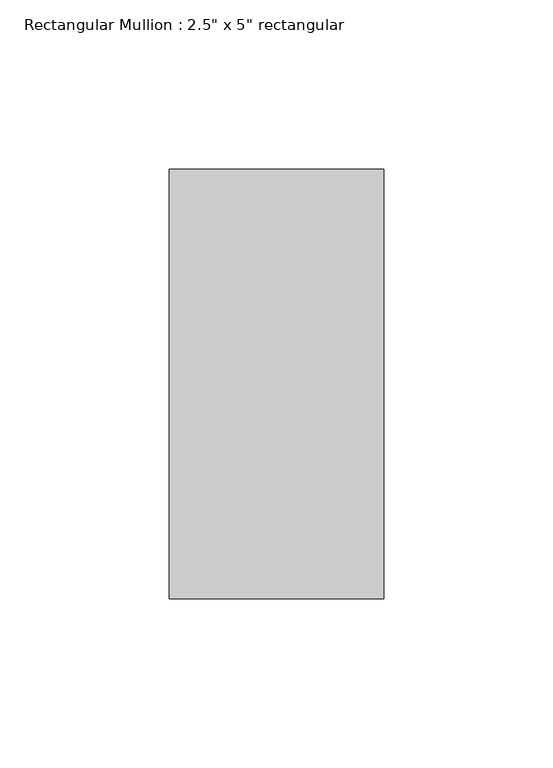
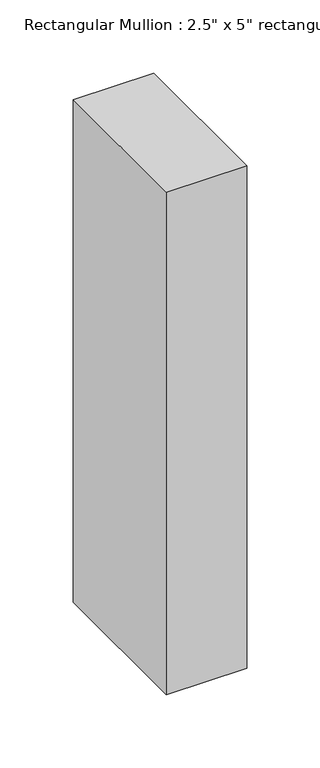
"""IFC4 building model written with IfcOpenShell, lengths in millimetres: member geometry."""

from ifc_helpers import new_model, si_unit, frame, origin, place, context, project, spatial, polyline, outline, extrude, source, transform, mapped, element, save


def member_05170f4c(model_context):
    return source(origin(), model_context, "Body", "SweptSolid", [
        extrude(outline(polyline([(0.0, 63.5), (0.0, -63.5), (-63.5, -63.5), (-63.5, 63.5), (0.0, 63.5)])), frame((0.0, 0.0, -419.0669271), z_axis=(0.0, 0.0, 1.0), x_axis=(1.0, 0.0, 0.0)), (0.0, 0.0, 1.0), 419.0669271),
    ])


if __name__ == "__main__":
    model = new_model("IFC4")
    model_context = context("Model", 3, world=origin())
    ifc_project = project(units=[si_unit("LENGTHUNIT", "METRE", prefix="MILLI")], contexts=[model_context])
    site = spatial("IfcSite", under=ifc_project)
    building = spatial("IfcBuilding", under=site)
    placement = place(None, origin())
    member_shape = member_05170f4c(model_context)
    element("IfcMember", 1, ObjectType="Rectangular Mullion : 2.5\" x 5\" rectangular", at=placement, inside=building, context=model_context, shape_type="MappedRepresentation", body=[
        mapped(member_shape, transform((0.0, 0.0, 0.0), x_axis=(1.0, 0.0, 0.0), y_axis=(0.0, 1.0, 0.0), z_axis=(0.0, 0.0, 1.0))),
    ])
    save(model, "model.ifc")

# Revit data of these elements
# Type "Rectangular Mullion : 2.5\" x 5\" rectangular"
#   built-in parameter 1007304 = 0.416667 (stored number, unit not read)
#   built-in parameter 1007301 = 0.104167 (stored number, unit not read)
#   built-in parameter 1007300 = 0.104167 (stored number, unit not read)
# Element 1 (IfcMember, "Rectangular Mullion : 2.5\" x 5\" rectangular")
#   Materials on its faces: "Aluminum"
# Materials
#   "Aluminum": class "Metal", colour RGB 247 247 247, transparency 0, Description = "Aluminum 6061", Cost = 0
